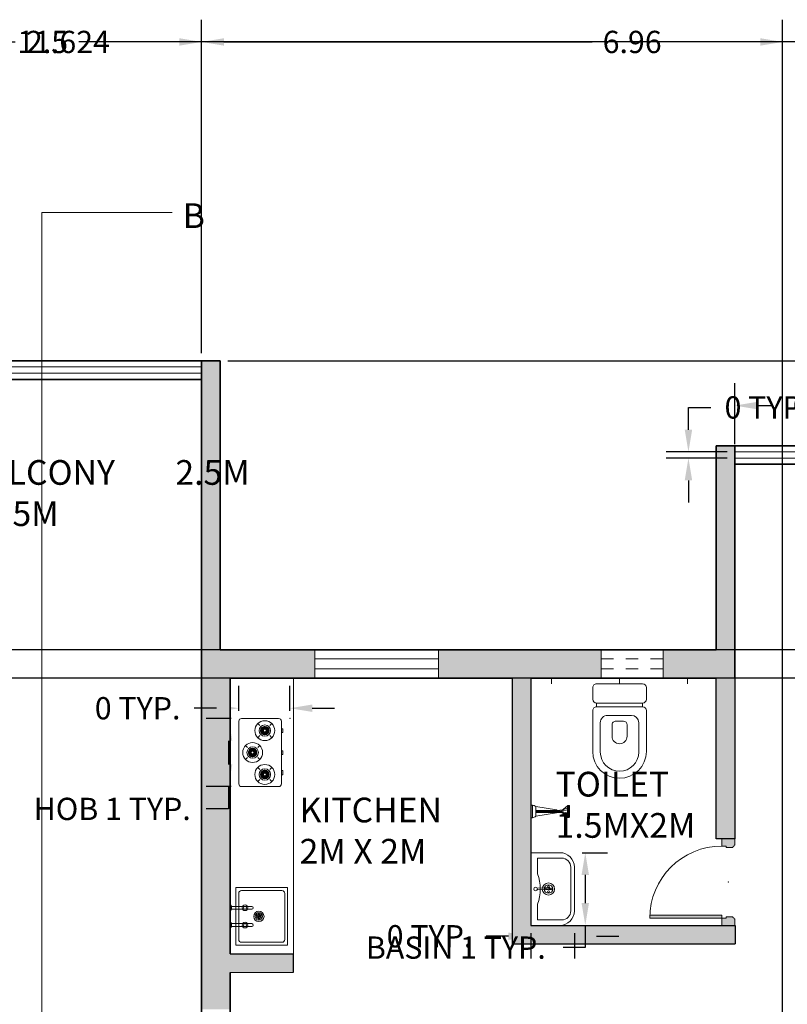
# Model space of a CAD drawing. Units: metres. Extents: x 2031 to 2061.8, y 1886.4 to 1909.8.
# Tile 10 of 10: x 2045.9 to 2052.1, y 1901.9 to 1909.8. Entities that reach past the tile are written whole.
import ezdxf

# ---------------------------------------------------------------- set-up
doc = ezdxf.new("R2010")
doc.units = ezdxf.units.M
doc.linetypes.add('DASHED', pattern=[0.75, 0.5, -0.25])
for name, color, linetype, lineweight in [('A-ANNO-DIMS', 2, 'Continuous', 18), ('A-ANNO-SYMB', 7, 'Continuous', 18), ('A-AREA-IDEN', 7, 'Continuous', 18), ('A-EQPM', 8, 'Continuous', 18), ('A-FLOR-CASE', 8, 'Continuous', 18), ('A-FLOR-FIXT', 8, 'Continuous', 18), ('A-GLAZ-OVHD', 30, 'DASHED', 13), ('A-WALL-PATT', 252, 'Continuous', 13), ('doors & windows', 30, 'Continuous', 18), ('furniture', 24, 'Continuous', 13), ('grills', 5, 'Continuous', 13), ('inner walls', 4, 'Continuous', 25), ('windows', 30, 'Continuous', 18)]:
    doc.layers.add(name, color=color, linetype=linetype, lineweight=lineweight)
doc.layers.add('outer walls', color=1, linetype='Continuous', lineweight=35, plot=False)
doc.styles.get("Standard").update_dxf_attribs({"font": 'arial.ttf'})
doc.dimstyles.get("Standard").update_dxf_attribs({"dimtxt": 0.18, "dimasz": 0.18, "dimexe": 0.18, "dimexo": 0.0625, "dimgap": 0.09, "dimtad": 0, "dimtih": 1, "dimtoh": 1, "dimdec": 4, "dimzin": 0, "dimdsep": 46, "dimtxsty": 'Standard', "dimcen": 0.09, "dimadec": 0, "dimazin": 0, "dimtfac": 1, "dimtdec": 4, "dimtofl": 0, "dimtmove": 0, "dimatfit": 3, "dimfxl": 1, "dimtolj": 1, "dimtzin": 0, "dimarcsym": 0})

# ---------------------------------------------------------------- blocks, each defined once
blk = doc.blocks.new('commode')
for p, q in [((-7.091161676878982, 19.40883832311374), (-7.091161676878982, 8.608954493363852)), ((-5.091161676878982, 11.8123055313481), (-5.091161676878982, 19.56719258349039)), ((5.091161676893534, 11.8123055313481), (5.091161676893534, 19.56719258349039)), ((7.091161676893534, 19.40883832311374), (7.091161676893534, 8.608954493363852)), ((-1.999999999985448, 12.37086546904174), (-1.999999999985448, 15.37086546904174)), ((2.000000000014551, 12.37086546904174), (2.000000000014551, 15.37086546904174)), ((-0.999999999985448, 11.37086546904174), (1.000000000014551, 11.37086546904174)), ((-3.149721614536247, 9.870865469041746), (3.149721614565351, 9.870865469041746)), ((-7.091161676878982, 2.5), (-7.091161676878982, 5.608954493363853)), ((-6.091161676878982, 7.608954493363853), (6.091161676893534, 7.608954493363853)), ((-6.091161676878982, 6.608954493363853), (-6.091161676878982, 7.608954493363851)), ((-6.091161676878982, 6.608954493363853), (6.091161676893534, 6.608954493363853)), ((6.091161676893534, 7.608954493363854), (6.091161676893534, 6.608954493363853)), ((7.091161676893534, 2.5), (7.091161676893534, 5.608954493363853)), ((-18, 1.5), (-18, 0)), ((-6.091161676878982, 1.5), (6.091161676893534, 1.5)), ((0, 1.5), (0, 0)), ((18, 1.5), (18, 0))]:
    blk.add_line(p, q)
for centre, radius, start, end in [((7.276e-12, 19.40883832311374), 7.091161676886258, 0, 180), ((7.276e-12, 19.56719258349039), 5.091161676886258, 0, 180), ((7.276e-12, 15.37086546904174), 2, 0, 180), ((-3.149721614536247, 11.8123055313481), 1.941440062334415, 180, 270), ((-0.999999999985448, 12.37086546904174), 1, 180, 270), ((1.000000000014551, 12.37086546904174), 1, 270, 0), ((3.149721614565351, 11.8123055313481), 1.941440062334415, 270, 0), ((-6.091161676878982, 8.608954493363852), 1, 180, 270), ((6.091161676893534, 8.608954493363852), 1, 270, 0), ((-6.091161676878982, 5.608954493363853), 1, 90, 180), ((6.091161676893534, 5.608954493363853), 1, 0, 90), ((-6.091161676878982, 2.5), 1, 180, 270), ((6.091161676893534, 2.5), 1, 270, 0)]:
    blk.add_arc(centre, radius, start, end)
blk = doc.blocks.new('sink')
for p, q in [((0, 0), (-22.00000000000001, 0)), ((0, 0), (0, 0)), ((-20.00000000000023, -2.999999999999995), (-2.000000000000178, -3)), ((-19.99999999999959, -22.99999999999988), (-20.00000000000023, -2.999999999999995)), ((-2.000000000000178, -3), (-1.999999999999543, -22.99999999999988)), ((-18.99999999999966, -20.99999999999994), (-19.00000000000017, -4.999999999999996)), ((-18.00000000000017, -3.999999999999996), (-4.000000000000113, -3.999999999999999)), ((-3.000000000000114, -5), (-2.999999999999607, -20.99999999999988)), ((-0.5000000000000026, -9.499999999999813), (-7.500000000000004, -9.499999999999812)), ((-0.5000000000000026, -9.499999999999813), (-0.5000000000000028, -10.49999999999981)), ((-2.4e-15, -8.999999999999813), (-2.9e-15, -10.99999999999981)), ((-0.5000000000000028, -10.49999999999981), (-7.500000000000004, -10.49999999999981)), ((-0.500000000000004, -15.49999999999981), (-7.500000000000005, -15.49999999999981)), ((-0.5000000000000044, -16.49999999999981), (-7.500000000000005, -16.49999999999981)), ((-0.500000000000004, -15.49999999999981), (-0.5000000000000044, -16.49999999999981)), ((-3.9e-15, -14.99999999999981), (-4.4e-15, -16.99999999999981)), ((-19.99999999999959, -22.99999999999988), (-1.999999999999543, -22.99999999999988)), ((-17.99999999999966, -21.99999999999988), (-3.999999999999607, -21.99999999999989))]:
    blk.add_line(p, q)
for centre, radius in [((-5.180961460384426, -9.999999999999812), 1), ((-5.180961460384426, -9.999999999999812), 0.5), ((-10.00000000000014, -12.99999999999968), 1.794435724606955), ((-10.00000000000014, -12.99999999999968), 1.294435724606955), ((-10.66093109696162, -12.61841125325318), 0.25), ((-10.66093109696162, -13.38158874674618), 0.25), ((-10.00000000000014, -12.23682250650668), 0.25), ((-10.00000000000014, -12.99999999999968), 0.25), ((-10.00000000000014, -13.76317749349269), 0.25), ((-9.33906890303867, -12.61841125325318), 0.25), ((-9.33906890303867, -13.38158874674618), 0.25), ((-5.180961460384427, -15.99999999999981), 1), ((-5.180961460384427, -15.99999999999981), 0.5)]:
    blk.add_circle(centre, radius)
for centre, radius, start, end in [((-18.00000000000017, -4.999999999999996), 1, 89.99999999999999, 180), ((-4.000000000000115, -5), 1, 0, 89.99999999999999), ((-7.500000000000004, -9.999999999999812), 0.5, 89.99999999999999, 270), ((0.010449978117122, -9.510449978116938), 0.5105569333604445, 91.17280055555744, 178.8271994444424), ((0.0104499781171218, -10.48955002188269), 0.5105569333604445, 181.1728005555574, 268.8271994444423), ((-7.500000000000005, -15.99999999999981), 0.5, 89.99999999999999, 270), ((0.0104499781171206, -15.51044997811693), 0.5105569333604445, 91.17280055555744, 178.8271994444424), ((0.0104499781171203, -16.48955002188269), 0.5105569333604445, 181.1728005555573, 268.8271994444423), ((-17.99999999999966, -20.99999999999988), 1, 180, 270), ((-3.999999999999607, -20.99999999999988), 1, 270, 0)]:
    blk.add_arc(centre, radius, start, end)
blk = doc.blocks.new('stove')
at = {"layer": 'furniture'}
h = blk.add_hatch(dxfattribs=at)
h.set_pattern_fill('HEX', color=256, angle=180, style=0)
h.set_pattern_definition([(360, (23.99999999999982, 24.99999999999816), (1e-16, 0.216506351), [0.125, -0.25]), (119.9999999999999, (23.99999999999982, 24.99999999999816), (-0.1875000000466704, -0.1082531754999999), [0.1249999999999998, -0.2499999999999996]), (59.99999999999994, (24.12499999999982, 24.99999999999816), (-0.1875000000466704, 0.1082531755000001), [0.125, -0.25])])
h.paths.add_polyline_path([(10.36428182591571, 19.71316705046143, 1), (7.364281825915714, 19.71316705046143, 1)])
h.paths.add_polyline_path([(9.364281825915715, 19.71316705046143, -1), (8.364281825915715, 19.71316705046143, -1)], flags=16)
h = blk.add_hatch(dxfattribs=at)
h.set_pattern_fill('HEX', color=256, angle=180, style=0)
h.set_pattern_definition([(180, (-2.000000000000001, 6.713167050462818), (-1e-16, -0.216506351), [0.125, -0.25]), (300, (-2.000000000000001, 6.713167050462818), (0.1875000000466704, 0.1082531754999999), [0.1249999999999999, -0.2499999999999998]), (239.9999999999999, (-2.125000000000001, 6.713167050462818), (0.1875000000466704, -0.1082531755000001), [0.125, -0.25])])
h.paths.add_polyline_path([(14.6357181740841, 11.99999999999954, 1), (11.6357181740841, 11.99999999999954, 1)])
h.paths.add_polyline_path([(12.6357181740841, 11.99999999999954, -1), (13.6357181740841, 11.99999999999954, -1)], flags=16)
h = blk.add_hatch(dxfattribs=at)
h.set_pattern_fill('HEX', color=256, angle=180, style=0)
h.set_pattern_definition([(360, (23.99999999999982, -0.9999999999999342), (-1e-16, -0.216506351), [0.125, -0.25]), (239.9999999999999, (23.99999999999982, -0.9999999999999342), (-0.1875000000466704, 0.1082531755), [0.1249999999999999, -0.2499999999999998]), (300, (24.12499999999982, -0.9999999999999342), (-0.1875000000466704, -0.1082531755), [0.125, -0.2499999999999999])])
h.paths.add_polyline_path([(10.36428182591571, 4.2868329495368, 1), (7.364281825915714, 4.2868329495368, 1)])
h.paths.add_polyline_path([(9.364281825915715, 4.2868329495368, -1), (8.364281825915715, 4.2868329495368, -1)], flags=16)
for p, q in [((3, 1.000000000000003), (3.000000000000007, 22.99999999999909)), ((4.000000000000007, 23.99999999999909), (17, 23.99999999999908)), ((6.389408091762671, 22.18804078461422), (7.09651487294905, 21.48093400342751)), ((10.6320487788818, 21.48093400342809), (11.33915556006851, 22.18804078461447)), ((18, 22.99999999999908), (18, 0.9999999999991327)), ((3.000000000000007, 19.86017834974973), (2.500000000000003, 19.86017834974973)), ((2.500000000000003, 19.86017834974973), (2.500000000000003, 18.36017834974973)), ((2.500000000000003, 18.36017834974973), (3.000000000000003, 18.36017834974973)), ((6.389408091762675, 17.23829331630864), (7.096514872949061, 17.94540009749535)), ((10.63204877888179, 17.94540009749477), (11.3391555600685, 17.23829331630838)), ((11.36795122111803, 13.7677669529662), (10.66084443993131, 14.47487373415259)), ((15.61059190823715, 14.47487373415233), (14.90348512705075, 13.76776695296562)), ((2.500000000000003, 12.64999999999954), (2.500000000000003, 11.34999999999955)), ((3.000000000000003, 12.64999999999954), (2.500000000000003, 12.64999999999954)), ((2.500000000000003, 11.34999999999955), (3.000000000000003, 11.34999999999955)), ((11.36795122111803, 10.23223304703288), (10.66084443993131, 9.525126265846504)), ((15.61059190823714, 9.525126265846753), (14.90348512705077, 10.23223304703346)), ((2.500000000000003, 4.936832949536799), (2.500000000000003, 3.636832949536802)), ((3.000000000000003, 4.936832949536799), (2.500000000000003, 4.936832949536799)), ((2.500000000000003, 3.636832949536802), (3.000000000000003, 3.636832949536802)), ((6.389408091762671, 6.761706683689592), (7.096514872949061, 6.054599902502877)), ((10.63204877888178, 6.05459990250346), (11.3391555600685, 6.761706683689842)), ((16.99999999999994, -8.669e-13), (3.999999999999946, 3.6e-15)), ((6.389408091762668, 1.811959215384014), (7.096514872949043, 2.519065996570723)), ((10.63204877888179, 2.519065996570138), (11.3391555600685, 1.81195921538376))]:
    blk.add_line(p, q, dxfattribs=at)
for centre, radius in [((8.864281825915715, 19.71316705046143), 3.499999999999999), ((8.864281825915715, 19.71316705046143), 1.999999999999999), ((8.864281825915715, 19.71316705046143), 1.5), ((8.864281825915715, 19.71316705046143), 0.5000000000000004), ((13.1357181740841, 11.99999999999954), 3.499999999999999), ((13.1357181740841, 11.99999999999954), 1.999999999999999), ((13.1357181740841, 11.99999999999954), 1.5), ((13.1357181740841, 11.99999999999954), 0.5000000000000004), ((8.864281825915715, 4.286832949536801), 3.499999999999999), ((8.864281825915715, 4.2868329495368), 1.999999999999999), ((8.864281825915715, 4.2868329495368), 1.5), ((8.864281825915715, 4.2868329495368), 0.5000000000000004)]:
    blk.add_circle(centre, radius, dxfattribs=at)
for centre, start, end in [((4.000000000000007, 22.99999999999909), 90, 180), ((17, 22.99999999999908), 0, 90), ((4, 1.000000000000003), 180, 269.9999999999968), ((17, 0.9999999999991331), 269.9999999999968, 0)]:
    blk.add_arc(centre, 1, start, end, dxfattribs=at)
at = {"layer": 'furniture', "ltscale": 9}
blk.add_point((0, 0), dxfattribs=at)
blk = doc.blocks.new('D2')
at = {"layer": 'doors & windows'}
h = blk.add_hatch(dxfattribs=at)
h.set_pattern_fill('DOTS', color=256, scale=2, angle=180, style=0)
h.set_pattern_definition([(180, (0, -3.999999999998181), (-0.0625, -0.125), [0, -0.125])])
h.paths.add_polyline_path([(2.5, 1.819e-12), (3.5, 1.819e-12), (3.500000000001818, 24.97999199359535, 0.0100030022021123), (2.500000000001818, 25.00000000000182)])
h = blk.add_hatch(dxfattribs=at)
h.set_pattern_fill('DOTS', color=256, scale=2, angle=180, style=0)
h.set_pattern_definition([(180, (0, 0), (-0.0625, -0.125), [0, -0.125])])
edge = h.paths.add_edge_path()
edge.add_line((27.50000000000182, 1.819e-12), (27.50000000000182, -1.499999999998181))
edge.add_line((27.50000000000182, -1.499999999998181), (27.00000000000157, -1.499999999998181))
edge.add_line((27.00000000000157, -1.499999999998181), (27.00000000000039, -3.749999999998181))
edge.add_line((27.00000000000039, -3.749999999998181), (27.25, -3.749999999998181))
edge.add_arc((27.75893604593965, -3.741063954058532), 0.5090144907305875, 181.0059124648427, 268.9940875351573)
edge.add_line((27.75, -4.249999999998181), (27.75, -4.499999999998181))
edge.add_line((27.75, -4.499999999998181), (30.00000000000182, -4.499999999998181))
edge.add_line((30.00000000000182, -4.499999999998181), (30.00000000000182, 0))
edge.add_line((30.00000000000182, 0), (27.50000000000182, 1.819e-12))
edge = h.paths.add_edge_path()
edge.add_line((2.5, -1.499999999998181), (2.5, 1.819e-12))
edge.add_line((2.5, 1.819e-12), (1.819e-12, 0))
edge.add_line((1.819e-12, 0), (0, -4.499999999998181))
edge.add_line((0, -4.499999999998181), (2.250000000001548, -4.499999999998181))
edge.add_line((2.250000000001548, -4.499999999998181), (2.250000000001548, -4.249999999998181))
edge.add_arc((2.2410639540619, -3.741063954058532), 0.5090144907305875, 271.0059124648427, 358.9940875351573)
edge.add_line((2.750000000001548, -3.749999999998181), (3, -3.749999999998181))
edge.add_line((3, -3.749999999998181), (3, -1.499999999998181))
edge.add_line((3, -1.499999999998181), (2.5, -1.499999999998181))
for p, q in [((1.819e-12, 0), (0, -4.499999999998181)), ((30.00000000000182, 0), (30.00000000000182, -4.499999999998181))]:
    blk.add_line(p, q)
blk.add_lwpolyline([(3.5, 1.819e-12), (3.500000000001818, 25.00000000000182), (2.500000000001818, 25.00000000000182), (2.5, 1.819e-12)], close=True, dxfattribs=at)
for points in [[(3, -3.749999999998181), (3, -1.499999999998181), (2.5, -1.499999999998181), (2.5, 1.819e-12), (1.819e-12, 0)], [(27.00000000000039, -3.749999999998181), (27.00000000000182, -1.499999999998181), (27.50000000000182, -1.499999999998181), (27.50000000000182, 1.819e-12), (30, 0)], [(0, -4.499999999998181), (2.250000000001548, -4.499999999998181)], [(30, -4.499999999998181), (27.75, -4.499999999998181)]]:
    blk.add_lwpolyline(points, dxfattribs=at)
for points in [[(2.250000000001548, -4.499999999998181), (2.250000000001548, -4.249999999998181, 0.4039662087126686), (2.750000000001548, -3.749999999998181), (3.000000000001548, -3.749999999998181)], [(27.75, -4.499999999998181), (27.75, -4.249999999998181, -0.4039662087126686), (27.25, -3.749999999998181), (27, -3.749999999998181)]]:
    blk.add_lwpolyline(points, format="xyb", dxfattribs=at)
at = {"layer": 'doors & windows', "ltscale": 6}
blk.add_arc((2.5, 1.819e-12), 25, 0, 90, dxfattribs=at)
at = {"layer": 'doors & windows'}
blk.add_point((15, -2.24999999999909), dxfattribs=at)
blk = doc.blocks.new('wash basin 1')
for p, q in [((-8.5, 8.5), (-1.851811242548834, 8.500000000000004)), ((2.4e-15, 10), (-8, 10)), ((-1.851811242548834, 8.500000000000004), (-1.851811242548897, 4.188089367671713)), ((2.4e-15, 10), (-2.4e-15, -10)), ((-12, 6), (-12, -6.000000000000001)), ((-11, 6), (-11, -6.000000000000001)), ((-1.851811242548729, -8.5), (-1.851811242548728, -4.188089367671126)), ((-8.500000000000002, -8.500000000000002), (-1.851811242548729, -8.5)), ((-2.4e-15, -10), (-8.000000000000002, -10))]:
    blk.add_line(p, q)
blk.add_lwpolyline([(-1.829996854681013, 0.1082389988048371), (-5.253671435714977, 0.2462926470149123), (-5.229221238307189, -0.3815455523157976), (-1.804400006573047, -0.1898693366394459)])
for centre, radius in [((-4.868871099337752, 1.8e-15), 1.677439688297454), ((-4.868871099337752, 1.8e-15), 1.177439688297454), ((-5.631604960595723, 1.8e-15), 0.25), ((-4.873580145140294, 0.7523876361110525), 0.25), ((-4.868871099337752, 1.8e-15), 0.25), ((-4.194973017078154, 1.8e-15), 0.25), ((-1.341853106244229, 7.967e-13), 0.5), ((-4.868871099337752, -0.7188855560125376), 0.25)]:
    blk.add_circle(centre, radius)
for centre, radius, start, end in [((-8, 6), 4, 90, 180), ((-8.5, 6), 2.5, 90, 180), ((8.8933346853213, 5.103e-13), 11.53248687676786, 158.7058692194464, 201.2941307805559), ((-8.000000000000002, -6.000000000000001), 4, 180, 270), ((-8.500000000000002, -6.000000000000001), 2.5, 180, 270)]:
    blk.add_arc(centre, radius, start, end)
blk = doc.blocks.new('tap & shower')
for p, q in [((1.708172111072059, 0), (-1.708172111072059, 0)), ((-1.708172111072059, 0), (-1.708166955903891, -0.5000109134438162)), ((1.708172111072059, 0), (1.708172111072059, -0.5)), ((1.708172111072059, -0.5), (-1.708172111072059, -0.5)), ((1.30544807404803, -1.402724037024029), (-1.30544807404803, -1.402724037024029)), ((-1.305442878530783, -1.402734990816952), (-0.3920875420875518, -6.99797979797978)), ((-0.3171055409637802, -0.5), (0.3171055409637802, -0.5)), ((-0.269360269360277, -7.941077441077368), (-0.269360269360277, -1.402724037024029)), ((-0.2154882154882216, -7.941077441077368), (-0.2154882154882216, -1.402724037024029)), ((-0.1616161616161662, -7.941077441077368), (-0.1616161616161662, -1.402724037024029)), ((0, -8.47979797979798), (0, -1.402724037024029)), ((0.1616161616161662, -7.941077441077425), (0.1616161616161662, -1.402724037024029)), ((0.2154882154882216, -7.941077441077425), (0.2154882154882216, -1.402724037024029)), ((0.269360269360277, -7.941077441077425), (0.269360269360277, -1.402724037024029)), ((0.3920875420875234, -6.99797979797978), (1.30544807404803, -1.402724037024029)), ((-0.3232323232323324, -7.941077441077368), (0.3232323232323324, -7.941077441077482)), ((-0.3232323232323324, -8.47979797979798), (-0.3232323232323324, -7.941077441077368)), ((0.3232323232323324, -8.47979797979798), (0.3232323232323324, -7.941077441077482)), ((-1.616161616161605, -10.36531986531986), (-1.616161616161605, -10.09595959595958)), ((-1.481481481481495, -9.961279461279444), (-0.269360269360277, -8.47979797979798)), ((-1.481481481481495, -9.961279461279444), (1.481481481481466, -9.961279461279444)), ((-1.481481481481495, -10.5), (-1.481481481481495, -9.961279461279444)), ((-1.481481481481495, -10.5), (1.481481481481466, -10.5)), ((-1.427609427609439, -10.5), (-1.427609427609439, -9.961279461279444)), ((-1.373737373737384, -10.5), (-1.373737373737384, -9.961279461279444)), ((-1.319865319865328, -10.5), (-1.319865319865328, -9.961279461279444)), ((-1.265993265993273, -10.5), (-1.265993265993273, -9.961279461279444)), ((-1.212121212121218, -10.5), (-1.212121212121218, -9.961279461279444)), ((-1.158249158249162, -10.5), (-1.158249158249162, -9.961279461279444)), ((-1.104377104377107, -10.5), (-1.104377104377107, -9.961279461279444)), ((-1.050505050505051, -10.5), (-1.050505050505051, -9.961279461279444)), ((-0.9966329966329965, -10.5), (-0.9966329966329965, -9.961279461279444)), ((-0.2141589775469583, -8.47979797979798), (-0.9427609427609411, -9.961279461279444)), ((-0.9427609427609411, -10.5), (-0.9427609427609411, -9.961279461279444)), ((-0.8888888888888857, -10.5), (-0.8888888888888857, -9.961279461279444)), ((-0.8350168350168303, -10.5), (-0.8350168350168303, -9.961279461279444)), ((-0.781144781144775, -10.5), (-0.781144781144775, -9.961279461279444)), ((-0.7272727272727196, -10.5), (-0.7272727272727196, -9.961279461279444)), ((-0.6734006734006642, -10.5), (-0.6734006734006642, -9.961279461279444)), ((-0.6195286195286088, -10.5), (-0.6195286195286088, -9.961279461279444)), ((-0.5656565656565534, -10.5), (-0.5656565656565534, -9.961279461279444)), ((-0.5117845117845264, -10.5), (-0.5117845117845264, -9.961279461279444)), ((-0.457912457912471, -10.5), (-0.457912457912471, -9.961279461279444)), ((-0.0948641971181132, -8.47979797979798), (-0.4040404040404156, -9.961279461279444)), ((-0.4040404040404156, -10.5), (-0.4040404040404156, -9.961279461279444)), ((-0.3501683501683601, -10.5), (-0.3501683501683601, -9.961279461279444)), ((-0.3232323232323324, -8.47979797979798), (0.3232323232323324, -8.47979797979798)), ((-0.2962962962963047, -10.5), (-0.2962962962963047, -9.961279461279444)), ((-0.2424242424242493, -10.5), (-0.2424242424242493, -9.961279461279444)), ((-0.1885521885521939, -10.5), (-0.1885521885521939, -9.961279461279444)), ((-0.1346801346801385, -10.5), (-0.1346801346801385, -9.961279461279444)), ((-0.0808080808080831, -10.5), (-0.0808080808080831, -9.961279461279444)), ((-0.0269360269360277, -10.5), (-0.0269360269360277, -9.961279461279444)), ((0.0269360269360277, -10.5), (0.0269360269360277, -9.961279461279444)), ((0.0808080808080831, -10.5), (0.0808080808080831, -9.961279461279444)), ((0.0948641971181132, -8.47979797979798), (0.4040404040404156, -9.961279461279444)), ((0.1346801346801385, -10.5), (0.1346801346801385, -9.961279461279444)), ((0.1885521885521939, -10.5), (0.1885521885521939, -9.961279461279444)), ((0.2141589775469583, -8.47979797979798), (0.9427609427609411, -9.961279461279444)), ((0.2424242424242493, -10.5), (0.2424242424242493, -9.961279461279444)), ((1.481481481481466, -9.961279461279444), (0.269360269360277, -8.47979797979798)), ((0.2962962962963047, -10.5), (0.2962962962963047, -9.961279461279444)), ((0.3501683501683601, -10.5), (0.3501683501683601, -9.961279461279444)), ((0.4040404040404156, -10.5), (0.4040404040404156, -9.961279461279444)), ((0.4579124579124425, -10.5), (0.4579124579124425, -9.961279461279444)), ((0.5117845117844979, -10.5), (0.5117845117844979, -9.961279461279444)), ((0.5656565656565534, -10.5), (0.5656565656565534, -9.961279461279444)), ((0.6195286195286088, -10.5), (0.6195286195286088, -9.961279461279444)), ((0.6734006734006642, -10.5), (0.6734006734006642, -9.961279461279444)), ((0.7272727272727196, -10.5), (0.7272727272727196, -9.961279461279444)), ((0.781144781144775, -10.5), (0.781144781144775, -9.961279461279444)), ((0.8350168350168303, -10.5), (0.8350168350168303, -9.961279461279444)), ((0.8888888888888857, -10.5), (0.8888888888888857, -9.961279461279444)), ((0.9427609427609411, -10.5), (0.9427609427609411, -9.961279461279444)), ((0.9966329966329965, -10.5), (0.9966329966329965, -9.961279461279444)), ((1.050505050505051, -10.5), (1.050505050505051, -9.961279461279444)), ((1.104377104377107, -10.5), (1.104377104377107, -9.961279461279444)), ((1.158249158249162, -10.5), (1.158249158249162, -9.961279461279444)), ((1.212121212121218, -10.5), (1.212121212121218, -9.961279461279444)), ((1.265993265993273, -10.5), (1.265993265993273, -9.961279461279444)), ((1.319865319865328, -10.5), (1.319865319865328, -9.961279461279444)), ((1.373737373737384, -10.5), (1.373737373737384, -9.961279461279444)), ((1.427609427609439, -10.5), (1.427609427609439, -9.961279461279444)), ((1.481481481481466, -10.5), (1.481481481481466, -9.961279461279444)), ((1.616161616161605, -10.36531986531986), (1.616161616161605, -10.09595959595958))]:
    blk.add_line(p, q)
for centre, radius, start, end in [((-0.0174713202327155, -0.2869501082291208), 1.704067674476668, 187.1825297220346, 220.9027681176297), ((0.0174793747132753, -0.2869501082291208), 1.704067674476639, 319.0972318823703, 352.8174702779653), ((0, -6.985663239740574), 0.3922809430333202, 181.7992278553774, 358.2007721446227), ((-1.481481481481495, -10.09595959595958), 0.1346801346801346, 90, 180), ((-1.481481481481495, -10.36531986531986), 0.1346801346801346, 180, 270), ((1.481481481481466, -10.09595959595958), 0.1346801346801346, 0, 90), ((1.481481481481466, -10.36531986531986), 0.1346801346801346, 270, 0)]:
    blk.add_arc(centre, radius, start, end)
blk = doc.blocks.new('WIN-1000')
for p, q in [((2.274e-13, 0), (0, 0.2299999999997908)), ((1.000000000000227, 9.095e-13), (1, 0.2300000000007003)), ((2.274e-13, 0.1549999999997453), (1.000000000000227, 0.1549999999997453)), ((2.274e-13, 0.0749999999998181), (1.000000000000227, 0.0749999999998181))]:
    blk.add_line(p, q)
blk = doc.blocks.new('BALCONY-GUARD-2500')
for p, q in [((4.547e-13, 0.0500000000010914), (2.5, 0.0500000000006367)), ((4.547e-13, 6.821e-13), (2.5, 4.547e-13))]:
    blk.add_line(p, q)
blk = doc.blocks.new('*D22')
at = {"layer": 'A-ANNO-DIMS', "color": 0, "lineweight": -2, "transparency": 16777216}
for p, q in [((2051.65388605158, 1906.406583869398), (2051.65388605158, 1906.899083869398)), ((2054.15388605158, 1906.406583869398), (2054.15388605158, 1906.899083869398)), ((2051.83388605158, 1906.719083869398), (2051.958210744622, 1906.719083869398)), ((2053.97388605158, 1906.719083869398), (2053.849561358537, 1906.719083869398))]:
    blk.add_line(p, q, dxfattribs=at)
at = {"layer": 'A-ANNO-DIMS', "color": 0, "transparency": 16777216}
for points in [[(2051.83388605158, 1906.749083869398), (2051.83388605158, 1906.689083869398), (2051.65388605158, 1906.719083869398)], [(2053.97388605158, 1906.749083869398), (2053.97388605158, 1906.689083869398), (2054.15388605158, 1906.719083869398)]]:
    blk.add_solid(points, dxfattribs=at)
at = {"layer": 'Defpoints', "color": 0, "transparency": 16777216}
for p in [(2054.15388605158, 1906.719083869398), (2051.65388605158, 1906.344083869398), (2054.15388605158, 1906.344083869398)]:
    blk.add_point(p, dxfattribs=at)
at = {"layer": 'A-ANNO-DIMS', "color": 0, "transparency": 16777216, "insert": (2052.90388605158, 1906.719083869398), "char_height": 0.18, "attachment_point": 5}
blk.add_mtext('\\A1;GUARD 3 TYP.', dxfattribs=at)
blk = doc.blocks.new('*D23')
at = {"layer": 'A-ANNO-DIMS', "color": 0, "lineweight": -2, "transparency": 16777216}
for p, q in [((2051.278886051582, 1906.524083869399), (2051.278886051582, 1906.704083869399)), ((2051.278886051582, 1906.704083869399), (2051.458886051582, 1906.704083869399)), ((2051.591386051581, 1906.344083869399), (2051.098886051582, 1906.344083869399)), ((2051.591386051581, 1906.294083869399), (2051.098886051582, 1906.294083869399)), ((2051.278886051582, 1906.114083869398), (2051.278886051582, 1905.934083869398))]:
    blk.add_line(p, q, dxfattribs=at)
at = {"layer": 'A-ANNO-DIMS', "color": 0, "transparency": 16777216}
for points in [[(2051.248886051581, 1906.524083869399), (2051.308886051582, 1906.524083869399), (2051.278886051582, 1906.344083869399)], [(2051.248886051581, 1906.114083869398), (2051.308886051582, 1906.114083869398), (2051.278886051582, 1906.294083869399)]]:
    blk.add_solid(points, dxfattribs=at)
at = {"layer": 'Defpoints', "color": 0, "transparency": 16777216}
for p in [(2051.278886051582, 1906.344083869399), (2051.653886051581, 1906.344083869399), (2051.653886051581, 1906.294083869399)]:
    blk.add_point(p, dxfattribs=at)
at = {"layer": 'A-ANNO-DIMS', "color": 0, "transparency": 16777216, "insert": (2051.917051126616, 1906.704083869398), "char_height": 0.18, "attachment_point": 5}
blk.add_mtext('\\A1;0 TYP.', dxfattribs=at)
blk = doc.blocks.new('*D26')
at = {"layer": 'A-ANNO-DIMS', "color": 0, "lineweight": -2, "transparency": 16777216}
for p, q in [((2047.581938181865, 1904.187832439381), (2047.381703543051, 1904.187832439381)), ((2047.561703543051, 1904.007832439382), (2047.561703543051, 1903.816268180623)), ((2047.581938181862, 1903.636268180623), (2047.381703543051, 1903.636268180623)), ((2047.561703543051, 1903.636268180623), (2047.561703543051, 1903.456268180623)), ((2047.561703543051, 1903.456268180623), (2047.381703543051, 1903.456268180623))]:
    blk.add_line(p, q, dxfattribs=at)
at = {"layer": 'A-ANNO-DIMS', "color": 0, "transparency": 16777216}
for points in [[(2047.531703543051, 1904.007832439382), (2047.591703543051, 1904.007832439382), (2047.561703543051, 1904.187832439381)], [(2047.531703543051, 1903.816268180623), (2047.591703543051, 1903.816268180623), (2047.561703543051, 1903.636268180623)]]:
    blk.add_solid(points, dxfattribs=at)
at = {"layer": 'Defpoints', "color": 0, "transparency": 16777216}
for p in [(2047.644438181865, 1904.187832439381), (2047.561703543051, 1903.636268180623), (2047.644438181862, 1903.636268180623)]:
    blk.add_point(p, dxfattribs=at)
at = {"layer": 'A-ANNO-DIMS', "color": 0, "transparency": 16777216, "insert": (2046.621000950964, 1903.456268180622), "char_height": 0.18, "attachment_point": 5}
blk.add_mtext('\\A1;HOB 1 TYP.', dxfattribs=at)
blk = doc.blocks.new('*D27')
at = {"layer": 'A-ANNO-DIMS', "color": 0, "lineweight": -2, "transparency": 16777216}
for p, q in [((2047.644438181865, 1904.250332439381), (2047.644438181865, 1904.450567078194)), ((2048.058111375933, 1904.250332439378), (2048.058111375935, 1904.450567078191)), ((2047.464438181865, 1904.270567078195), (2047.284438181864, 1904.270567078196)), ((2048.238111375933, 1904.27056707819), (2048.418111375934, 1904.270567078189))]:
    blk.add_line(p, q, dxfattribs=at)
at = {"layer": 'A-ANNO-DIMS', "color": 0, "transparency": 16777216}
for points in [[(2047.464438181865, 1904.300567078195), (2047.464438181864, 1904.240567078195), (2047.644438181865, 1904.270567078194)], [(2048.238111375934, 1904.30056707819), (2048.238111375933, 1904.240567078191), (2048.058111375933, 1904.270567078192)]]:
    blk.add_solid(points, dxfattribs=at)
at = {"layer": 'Defpoints', "color": 0, "transparency": 16777216}
for p in [(2047.644438181865, 1904.270567078194), (2047.644438181864, 1904.187832439381), (2048.058111375933, 1904.187832439378)]:
    blk.add_point(p, dxfattribs=at)
at = {"layer": 'A-ANNO-DIMS', "color": 0, "transparency": 16777216, "insert": (2046.82627310683, 1904.270567078196), "char_height": 0.18, "attachment_point": 5}
blk.add_mtext('\\A1;0 TYP.', dxfattribs=at)
blk = doc.blocks.new('*D28')
at = {"layer": 'A-ANNO-DIMS', "color": 0, "lineweight": -2, "transparency": 16777216}
for p, q in [((2050.419216339097, 1903.102134348595), (2050.624923910977, 1903.102134348595)), ((2050.444923910978, 1902.922134348595), (2050.444923910978, 1902.694083869401)), ((2050.419216339097, 1902.514083869401), (2050.624923910977, 1902.514083869401)), ((2050.444923910978, 1902.514083869401), (2050.444923910978, 1902.334083869401)), ((2050.444923910978, 1902.334083869401), (2050.264923910978, 1902.334083869401))]:
    blk.add_line(p, q, dxfattribs=at)
at = {"layer": 'A-ANNO-DIMS', "color": 0, "transparency": 16777216}
for points in [[(2050.414923910977, 1902.922134348595), (2050.474923910978, 1902.922134348595), (2050.444923910978, 1903.102134348595)], [(2050.414923910977, 1902.694083869401), (2050.474923910978, 1902.694083869401), (2050.444923910978, 1902.514083869401)]]:
    blk.add_solid(points, dxfattribs=at)
at = {"layer": 'Defpoints', "color": 0, "transparency": 16777216}
for p in [(2050.356716339098, 1903.102134348595), (2050.356716339098, 1902.514083869401), (2050.444923910978, 1902.514083869401)]:
    blk.add_point(p, dxfattribs=at)
at = {"layer": 'A-ANNO-DIMS', "color": 0, "transparency": 16777216, "insert": (2049.398505084238, 1902.3340838694), "char_height": 0.18, "attachment_point": 5}
blk.add_mtext('\\A1;BASIN 1 TYP.', dxfattribs=at)
blk = doc.blocks.new('*D29')
at = {"layer": 'A-ANNO-DIMS', "color": 0, "lineweight": -2, "transparency": 16777216}
for p, q in [((2049.82388605158, 1902.425876297521), (2049.643886051581, 1902.425876297521)), ((2050.00388605158, 1902.4515838694), (2050.00388605158, 1902.245876297521)), ((2050.356716339097, 1902.4515838694), (2050.356716339097, 1902.245876297521)), ((2050.536716339097, 1902.425876297521), (2050.716716339097, 1902.425876297521))]:
    blk.add_line(p, q, dxfattribs=at)
at = {"layer": 'A-ANNO-DIMS', "color": 0, "transparency": 16777216}
for points in [[(2049.82388605158, 1902.455876297521), (2049.82388605158, 1902.395876297521), (2050.00388605158, 1902.425876297521)], [(2050.536716339097, 1902.455876297521), (2050.536716339097, 1902.395876297521), (2050.356716339097, 1902.425876297521)]]:
    blk.add_solid(points, dxfattribs=at)
at = {"layer": 'Defpoints', "color": 0, "transparency": 16777216}
for p in [(2050.00388605158, 1902.5140838694), (2050.356716339097, 1902.5140838694), (2050.00388605158, 1902.425876297521)]:
    blk.add_point(p, dxfattribs=at)
at = {"layer": 'A-ANNO-DIMS', "color": 0, "transparency": 16777216, "insert": (2049.185720976546, 1902.425876297521), "char_height": 0.18, "attachment_point": 5}
blk.add_mtext('\\A1;0 TYP.', dxfattribs=at)
blk = doc.blocks.new('*D45')
at = {"layer": 'A-ANNO-DIMS', "color": 0, "lineweight": -2, "transparency": 16777216}
for p, q in [((2047.556386000001, 1907.081203000001), (2061.614374000002, 1907.081203000001)), ((2061.434374000002, 1906.901203000001), (2061.434374000002, 1897.862029637791)), ((2061.434374000002, 1888.459050000001), (2061.434374000002, 1897.498223362211)), ((2054.286386000001, 1888.279050000001), (2061.614374000002, 1888.279050000001))]:
    blk.add_line(p, q, dxfattribs=at)
at = {"layer": 'A-ANNO-DIMS', "color": 0, "transparency": 16777216}
for points in [[(2061.404374000002, 1906.901203000001), (2061.464374000002, 1906.901203000001), (2061.434374000002, 1907.081203000001)], [(2061.404374000002, 1888.459050000001), (2061.464374000002, 1888.459050000001), (2061.434374000002, 1888.279050000001)]]:
    blk.add_solid(points, dxfattribs=at)
at = {"layer": 'Defpoints', "color": 0, "transparency": 16777216}
for p in [(2047.493886000001, 1907.081203000001), (2061.434374000002, 1907.081203000001), (2054.223886000001, 1888.279050000001)]:
    blk.add_point(p, dxfattribs=at)
at = {"layer": 'A-ANNO-DIMS', "color": 0, "transparency": 16777216, "insert": (2061.434374000002, 1897.6801265), "char_height": 0.18, "attachment_point": 5}
blk.add_mtext('\\A1;18.802', dxfattribs=at)
blk = doc.blocks.new('*D48')
at = {"layer": 'A-ANNO-DIMS', "color": 0, "lineweight": -2, "transparency": 16777216}
for p, q in [((2044.843886, 1907.143703), (2044.843886, 1909.84065)), ((2047.343886, 1907.143703), (2047.343886, 1909.84065)), ((2045.023886, 1909.66065), (2045.837821879946, 1909.66065)), ((2047.163886, 1909.66065), (2046.349950120055, 1909.66065))]:
    blk.add_line(p, q, dxfattribs=at)
at = {"layer": 'A-ANNO-DIMS', "color": 0, "transparency": 16777216}
for points in [[(2045.023886, 1909.69065), (2045.023886, 1909.63065), (2044.843886, 1909.66065)], [(2047.163886, 1909.69065), (2047.163886, 1909.63065), (2047.343886, 1909.66065)]]:
    blk.add_solid(points, dxfattribs=at)
at = {"layer": 'Defpoints', "color": 0, "transparency": 16777216}
for p in [(2047.343886, 1909.66065), (2044.843886, 1907.081203), (2047.343886, 1907.081203)]:
    blk.add_point(p, dxfattribs=at)
at = {"layer": 'A-ANNO-DIMS', "color": 0, "transparency": 16777216, "insert": (2046.093886, 1909.66065), "char_height": 0.18, "attachment_point": 5}
blk.add_mtext('\\A1;2.5', dxfattribs=at)
blk = doc.blocks.new('*D49')
at = {"layer": 'A-ANNO-DIMS', "color": 0, "lineweight": -2, "transparency": 16777216}
for p, q in [((2047.343886, 1907.143703), (2047.343886, 1909.84065)), ((2054.303886, 1906.456584), (2054.303886, 1909.84065)), ((2047.523886, 1909.66065), (2050.499677268759, 1909.66065)), ((2054.123886000001, 1909.66065), (2051.148094731242, 1909.66065))]:
    blk.add_line(p, q, dxfattribs=at)
at = {"layer": 'A-ANNO-DIMS', "color": 0, "transparency": 16777216}
for points in [[(2047.523886, 1909.69065), (2047.523886, 1909.63065), (2047.343886, 1909.66065)], [(2054.123886000001, 1909.69065), (2054.123886000001, 1909.63065), (2054.303886, 1909.66065)]]:
    blk.add_solid(points, dxfattribs=at)
at = {"layer": 'Defpoints', "color": 0, "transparency": 16777216}
for p in [(2054.303886, 1909.66065), (2047.343886, 1907.081203), (2054.303886, 1906.394084)]:
    blk.add_point(p, dxfattribs=at)
at = {"layer": 'A-ANNO-DIMS', "color": 0, "transparency": 16777216, "insert": (2050.823886, 1909.66065), "char_height": 0.18, "attachment_point": 5}
blk.add_mtext('\\A1;6.96', dxfattribs=at)
blk = doc.blocks.new('*D58')
at = {"layer": 'A-ANNO-DIMS', "color": 0, "lineweight": -2, "transparency": 16777216}
for p, q in [((2040.415705, 1896.633713), (2040.415705, 1909.84065)), ((2052.040038, 1896.633713), (2052.040038, 1909.84065)), ((2040.595705, 1909.66065), (2045.773082959755, 1909.66065)), ((2051.860038, 1909.66065), (2046.682660040246, 1909.66065))]:
    blk.add_line(p, q, dxfattribs=at)
at = {"layer": 'A-ANNO-DIMS', "color": 0, "transparency": 16777216}
for points in [[(2040.595705, 1909.69065), (2040.595705, 1909.63065), (2040.415705, 1909.66065)], [(2051.860038, 1909.69065), (2051.860038, 1909.63065), (2052.040038, 1909.66065)]]:
    blk.add_solid(points, dxfattribs=at)
at = {"layer": 'Defpoints', "color": 0, "transparency": 16777216}
for p in [(2052.040038, 1909.66065), (2040.415705, 1896.571213), (2052.040038, 1896.571213)]:
    blk.add_point(p, dxfattribs=at)
at = {"layer": 'A-ANNO-DIMS', "color": 0, "transparency": 16777216, "insert": (2046.227871500001, 1909.66065), "char_height": 0.18, "attachment_point": 5}
blk.add_mtext('\\A1;11.624', dxfattribs=at)
blk = doc.blocks.new('*D60')
at = {"layer": 'A-ANNO-DIMS', "color": 0, "lineweight": -2, "transparency": 16777216}
for p, q in [((2031.744780000002, 1904.924084000001), (2031.744780000002, 1905.104084000001)), ((2056.161386000001, 1904.744084), (2031.564780000002, 1904.744084)), ((2055.931386000001, 1904.514084000001), (2031.564780000002, 1904.514084000001)), ((2031.744780000002, 1904.334084000001), (2031.744780000002, 1904.154084000001)), ((2031.744780000002, 1904.154084000001), (2031.564780000002, 1904.154084000001))]:
    blk.add_line(p, q, dxfattribs=at)
at = {"layer": 'A-ANNO-DIMS', "color": 0, "transparency": 16777216}
for points in [[(2031.714780000002, 1904.924084000001), (2031.774780000002, 1904.924084000001), (2031.744780000002, 1904.744084)], [(2031.714780000002, 1904.334084000001), (2031.774780000002, 1904.334084000001), (2031.744780000002, 1904.514084000001)]]:
    blk.add_solid(points, dxfattribs=at)
at = {"layer": 'Defpoints', "color": 0, "transparency": 16777216}
for p in [(2056.223886000001, 1904.744084), (2031.744780000002, 1904.514084000001), (2055.993886000001, 1904.514084000001)]:
    blk.add_point(p, dxfattribs=at)
at = {"layer": 'A-ANNO-DIMS', "color": 0, "transparency": 16777216, "insert": (2031.241001009552, 1904.154084), "char_height": 0.18, "attachment_point": 5}
blk.add_mtext('\\A1;0.23', dxfattribs=at)

msp = doc.modelspace()

# ---------------------------------------------------------------- hatches: boundary and pattern name
at = {"layer": 'A-WALL-PATT'}
h = msp.add_hatch(color=256, dxfattribs=at)
h.dxf.hatch_style = 1
h.paths.add_polyline_path([(2055.723886051581, 1899.601202985826), (2054.382747959846, 1899.601202985826), (2054.382747959846, 1900.884083869399), (2056.223886051581, 1900.884083869399), (2056.223886051581, 1902.238485983749), (2055.993886051581, 1902.238485983749), (2055.993886051581, 1901.1140838694), (2054.152747959847, 1901.1140838694), (2054.152747959847, 1899.684083882831), (2051.671801362485, 1899.684083882831), (2051.668720550386, 1900.463086761322), (2051.518721723415, 1900.462493543744), (2051.522127968044, 1899.601202985826), (2051.010160422872, 1899.601202985826), (2051.010160422872, 1899.371202985826), (2054.723886051581, 1899.371202985826), (2055.493886051581, 1899.371202985826), (2055.493886051581, 1895.571212564149), (2052.04003795628, 1895.571212564149), (2052.04003795628, 1895.334826264002), (2055.723886051581, 1895.334826264003)])
h.paths.add_polyline_path([(2056.223886051581, 1904.7440838694), (2054.30388605158, 1904.7440838694), (2054.30388605158, 1906.394083869399), (2054.15388605158, 1906.394083869399), (2054.15388605158, 1904.7440838694), (2052.35388605158, 1904.744083869399), (2052.35388605158, 1904.5140838694), (2055.993886051581, 1904.514083869399), (2055.993886051581, 1903.438485983748), (2056.223886051581, 1903.438485983749)])
h.paths.add_polyline_path([(2051.65388605158, 1906.394083869399), (2051.50388605158, 1906.394083869399), (2051.50388605158, 1904.7440838694), (2051.073484427694, 1904.7440838694), (2051.073484427694, 1904.5140838694), (2051.50388605158, 1904.5140838694), (2051.50388605158, 1903.2140838694), (2051.65388605158, 1903.2140838694), (2051.65388605158, 1904.514083869399), (2051.65388605158, 1904.744083869399)])
h.paths.add_polyline_path([(2050.573484427694, 1904.7440838694), (2049.259724738491, 1904.7440838694), (2049.259724738491, 1904.5140838694), (2049.85388605158, 1904.5140838694), (2049.85388605158, 1902.3640838694), (2051.657247644143, 1902.3640838694), (2051.656654421926, 1902.5140838694), (2051.54888605158, 1902.5140838694), (2050.00388605158, 1902.5140838694), (2050.00388605158, 1903.102134348594), (2050.00388605158, 1904.5140838694), (2050.573484427694, 1904.5140838694)])
h.paths.add_polyline_path([(2048.259724738491, 1904.7440838694), (2047.49388605158, 1904.7440838694), (2047.493886051581, 1907.081202972395), (2047.343886051582, 1907.081202972395), (2047.343886051581, 1901.835524324617), (2047.57388605158, 1901.835524324617), (2047.57388605158, 1902.134083869399), (2048.085735884881, 1902.134128710869), (2048.085735884882, 1902.284083869396), (2047.573886051581, 1902.2840838694), (2047.57388605158, 1904.5140838694), (2048.259724738491, 1904.5140838694)])
h.paths.add_polyline_path([(2047.57388605158, 1900.752643427613), (2047.34388605158, 1900.752643427612), (2047.34388605158, 1899.371202985826), (2047.57388605158, 1899.371202985826), (2047.57388605158, 1899.551202985826)])
h.paths.add_polyline_path([(2049.810160422872, 1899.601202985827), (2048.77388605158, 1899.601202985827), (2048.77388605158, 1899.371202985826), (2049.810160422872, 1899.371202985826)])

# ---------------------------------------------------------------- linework, layer by layer
at = {"layer": 'A-ANNO-SYMB'}
for p, q in [((2046.051788731911, 1887.95119549084), (2046.051788731911, 1908.279650182242)), ((2046.051788731911, 1908.279650182242), (2046.051788731911, 1908.279650182242)), ((2046.051788731911, 1908.279650182242), (2047.10641811258, 1908.279650182242))]:
    msp.add_line(p, q, dxfattribs=at)
at = {"layer": 'A-FLOR-CASE', "ltscale": 0.3}
msp.add_line((2048.085735884895, 1904.5140838694), (2048.085735884882, 1902.284083869397), dxfattribs=at)
at = {"layer": 'A-GLAZ-OVHD', "ltscale": 0.2}
for p, q in [((2050.573484427694, 1904.6690838694), (2051.073484427694, 1904.6690838694)), ((2050.573484427694, 1904.589083869399), (2051.073484427694, 1904.589083869399))]:
    msp.add_line(p, q, dxfattribs=at)
at = {"layer": 'inner walls'}
for p, q in [((2049.85388605158, 1904.5140838694), (2049.85388605158, 1902.3640838694)), ((2050.00388605158, 1904.5140838694), (2050.00388605158, 1902.5140838694)), ((2050.00388605158, 1902.5140838694), (2051.656654421926, 1902.5140838694)), ((2049.85388605158, 1902.3640838694), (2051.657247644144, 1902.3640838694)), ((2047.573886051581, 1902.2840838694), (2048.085735884882, 1902.284083869397)), ((2048.085735884881, 1902.134128710869), (2048.085735884882, 1902.284083869397)), ((2047.573886051581, 1902.134083869399), (2048.085735884881, 1902.134128710869))]:
    msp.add_line(p, q, dxfattribs=at)
for points in [[(2051.65388605158, 1904.514083869399), (2051.65388605158, 1903.2140838694), (2051.50388605158, 1903.2140838694), (2051.50388605158, 1904.5140838694)], [(2051.656654421926, 1902.5140838694), (2051.657247644143, 1902.3640838694)]]:
    msp.add_lwpolyline(points, dxfattribs=at)
at = {"layer": 'outer walls'}
for p, q in [((2044.843886051581, 1907.081202972395), (2047.493886051581, 1907.081202972395)), ((2047.343886051582, 1907.081202972395), (2047.34388605158, 1899.371202985826)), ((2047.493886051581, 1907.081202972395), (2047.49388605158, 1904.7440838694)), ((2044.843886051581, 1906.931202972395), (2047.343886051581, 1906.931202972395)), ((2051.50388605158, 1904.7440838694), (2051.50388605158, 1906.394083869399)), ((2051.50388605158, 1906.394083869399), (2054.30388605158, 1906.394083869399)), ((2051.65388605158, 1904.744083869399), (2051.65388605158, 1906.3940838694)), ((2051.65388605158, 1906.244083869399), (2054.15388605158, 1906.244083869399)), ((2047.493886051581, 1904.7440838694), (2051.50388605158, 1904.7440838694)), ((2051.65388605158, 1904.514083869399), (2051.65388605158, 1904.744083869399)), ((2047.573886051581, 1904.5140838694), (2049.85388605158, 1904.5140838694)), ((2047.57388605158, 1904.5140838694), (2047.573886051581, 1902.2840838694)), ((2050.00388605158, 1904.5140838694), (2051.50388605158, 1904.5140838694)), ((2047.57388605158, 1902.134083869399), (2047.57388605158, 1899.371202985826))]:
    msp.add_line(p, q, dxfattribs=at)
at = {"layer": 'windows'}
for p, q in [((2050.573484427694, 1904.5140838694), (2050.573484427694, 1904.7440838694)), ((2051.073484427694, 1904.5140838694), (2051.073484427694, 1904.7440838694))]:
    msp.add_line(p, q, dxfattribs=at)

# ---------------------------------------------------------------- block references
at = {"layer": 'A-EQPM', "xscale": 0.0229818441149355, "yscale": 0.0229818441149355, "zscale": 0.0229818441149355, "rotation": 179.9999999996526}
msp.add_blockref('stove', (2048.058111375933, 1904.187832439378), dxfattribs=at)
at = {"layer": 'A-FLOR-FIXT'}
for name, p, xscale, yscale, zscale, rotation in [('commode', (2050.722084892553, 1904.5140838694), 0.030558270807299, 0.030558270807299, 0.030558270807299, 180), ('tap & shower', (2050.003886051579, 1903.435651053365), -0.0297885069260649, 0.0297885069260649, 0.0297885069260649, 90), ('wash basin 1', (2050.00388605158, 1902.808109108997), 0.0294025239596969, 0.0294025239596969, 0.0294025239596969, 180), ('sink', (2047.573886051581, 1902.2840838694), 0.0232659015136525, 0.0232659015136525, 0.0232659015136525, 179.9999999996526)]:
    msp.add_blockref(name, p, dxfattribs=dict(at, xscale=xscale, yscale=yscale, zscale=zscale, rotation=rotation))
at = {"layer": 'doors & windows', "xscale": 0.0233333333333255, "yscale": 0.0233333333333255, "zscale": 0.0233333333333255, "rotation": 90.00000000000003}
msp.add_blockref('D2', (2051.54888605158, 1902.5140838694), dxfattribs=at)
at = {"layer": 'grills'}
for p in [(2044.843886051581, 1906.981202972394), (2051.65388605158, 1906.294083869397)]:
    msp.add_blockref('BALCONY-GUARD-2500', p, dxfattribs=at)
at = {"layer": 'windows', "rotation": 180}
msp.add_blockref('WIN-1000', (2049.259724738491, 1904.744083869399), dxfattribs=at)

# ---------------------------------------------------------------- texts
at = {"layer": 'A-ANNO-SYMB', "insert": (2047.190944202152, 1908.155561793653), "char_height": 0.2, "attachment_point": 7}
msp.add_mtext_dynamic_manual_height_columns('B', width=2.302330104705106, gutter_width=12.5, heights=[0], dxfattribs=at)
at = {"layer": 'A-AREA-IDEN', "attachment_point": 7}
for s, width, insert, char_height in [('BALCONY        2.5M X1.5M', 2.302330104705106, (2045.430973233493, 1905.744656013613), 0.2), ('TOILET\\P1.5MX2M', 1.594746697714981, (2050.204956578624, 1903.222610412209), 0.2000643999073453), ('KITCHEN \\P2M X 2M', 1.594746697714981, (2048.136131424042, 1903.013594329567), 0.2)]:
    msp.add_mtext_dynamic_manual_height_columns(s, width=width, gutter_width=12.5, heights=[0], dxfattribs=dict(at, insert=insert, char_height=char_height))

# ---------------------------------------------------------------- dimensions: what is measured, and where the dimension line sits
at = {"layer": 'A-ANNO-DIMS'}
for base, p1, p2, override, picture, middle in [((2052.040038, 1909.66065), (2040.415705, 1896.571213), (2052.040038, 1896.571213), {"dimdec": 3, "dimlfac": 1, "dimrnd": 0, "dimzin": 0, "dimdsep": 46, "dimlunit": 2}, '*D58', (2046.227871500001, 1909.66065)), ((2047.343886, 1909.66065), (2044.843886, 1907.081203), (2047.343886, 1907.081203), {"dimdec": 1, "dimlfac": 1, "dimrnd": 0, "dimzin": 0, "dimdsep": 46, "dimlunit": 2}, '*D48', (2046.093886, 1909.66065)), ((2054.303886, 1909.66065), (2047.343886, 1907.081203), (2054.303886, 1906.394084), {"dimdec": 2, "dimlfac": 1, "dimrnd": 0, "dimzin": 0, "dimdsep": 46, "dimlunit": 2}, '*D49', (2050.823886, 1909.66065))]:
    dim = msp.add_linear_dim(base=base, p1=p1, p2=p2, dimstyle='Standard', override=override, dxfattribs=at)
    dim.commit()
    dim.dimension.update_dxf_attribs({"geometry": picture, "text_midpoint": middle})
dim = msp.add_linear_dim(base=(2054.15388605158, 1906.719083869398), p1=(2051.65388605158, 1906.344083869398), p2=(2054.15388605158, 1906.344083869398), text='GUARD <> TYP.', dimstyle='Standard', override={"dimdec": 0, "dimlfac": 1, "dimrnd": 0, "dimzin": 0, "dimdsep": 46, "dimlunit": 2}, dxfattribs=at)
dim.commit()
dim.dimension.update_dxf_attribs({"geometry": '*D22', "text_midpoint": (2052.90388605158, 1906.719083869398)})
for base, p1, p2, override, picture, middle in [((2061.434374000002, 1907.081203000001), (2054.223886, 1888.27905), (2047.493886, 1907.081203), {"dimdec": 3, "dimlfac": 1, "dimrnd": 0, "dimzin": 0, "dimdsep": 46, "dimlunit": 2}, '*D45', (2061.434374000002, 1897.6801265)), ((2031.744780000002, 1904.514084000001), (2056.223886000001, 1904.744084), (2055.993886, 1904.514084), {"dimdec": 2, "dimlfac": 1, "dimrnd": 0, "dimzin": 0, "dimdsep": 46, "dimlunit": 2}, '*D60', (2031.241001009552, 1904.154084))]:
    dim = msp.add_linear_dim(base=base, p1=p1, p2=p2, angle=90, dimstyle='Standard', override=override, dxfattribs=at)
    dim.commit()
    dim.dimension.update_dxf_attribs({"geometry": picture, "text_midpoint": middle})
for base, p1, p2, angle, text, picture, middle in [((2051.278886051582, 1906.344083869399), (2051.65388605158, 1906.294083869397), (2051.65388605158, 1906.344083869398), 90, '<> TYP.', '*D23', (2051.917051126616, 1906.704083869398)), ((2047.644438181865, 1904.270567078194), (2048.058111375933, 1904.187832439378), (2047.644438181864, 1904.187832439381), 179.9999999996536, '<> TYP.', '*D27', (2046.82627310683, 1904.270567078196)), ((2047.561703543051, 1903.636268180623), (2047.644438181864, 1904.187832439381), (2047.644438181861, 1903.636268180622), 269.9999999996693, 'HOB <> TYP.', '*D26', (2046.621000950964, 1903.456268180622)), ((2050.444923910978, 1902.514083869401), (2050.356716339097, 1903.102134348594), (2050.356716339097, 1902.5140838694), 270, 'BASIN <> TYP.', '*D28', (2049.398505084238, 1902.3340838694)), ((2050.00388605158, 1902.425876297521), (2050.356716339097, 1902.5140838694), (2050.00388605158, 1902.5140838694), 180, '<> TYP.', '*D29', (2049.185720976546, 1902.425876297521))]:
    dim = msp.add_linear_dim(base=base, p1=p1, p2=p2, angle=angle, text=text, dimstyle='Standard', override={"dimdec": 0, "dimlfac": 1, "dimrnd": 0, "dimzin": 0, "dimdsep": 46, "dimlunit": 2}, dxfattribs=at)
    dim.commit()
    dim.dimension.update_dxf_attribs({"geometry": picture, "text_midpoint": middle})

doc.saveas('drawing.dxf')
